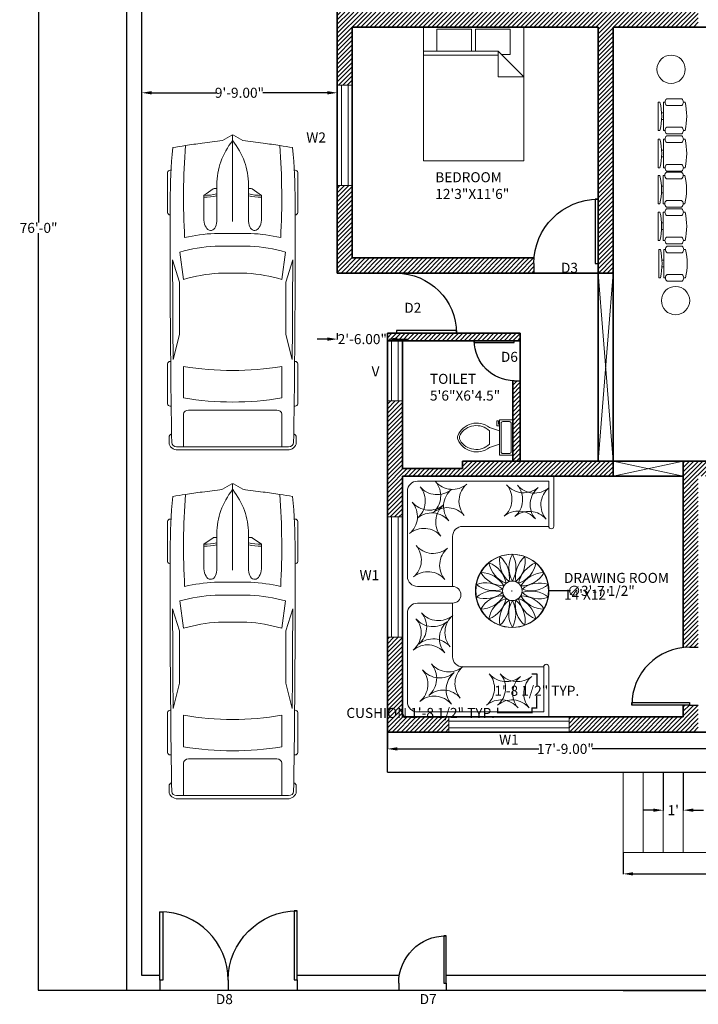
# Model space of a CAD drawing. Units: inches. Extents: x -57 to 1512, y -896 to 149.
# Tile 1 of 6: x -57 to 349, y -896 to -307. Entities that reach past the tile are written whole.
import ezdxf

# ---------------------------------------------------------------- set-up
doc = ezdxf.new("R2010")
doc.units = ezdxf.units.IN
doc.header["$MEASUREMENT"] = 0
doc.layers.get('Defpoints').update_dxf_attribs({"color": 9})
for name, color, linetype, lineweight in [('A-ANNO-DIMS', 2, 'Continuous', 18), ('A-ANNO-TEXT', 7, 'Continuous', 18), ('A-AREA-IDEN', 7, 'Continuous', 18), ('A-DOOR', 3, 'Continuous', 25), ('A-FLOR', 7, 'Continuous', 25), ('A-FLOR-FIXT', 9, 'Continuous', 18), ('A-FLOR-STRS', 7, 'Continuous', 18), ('A-FURN', 8, 'Continuous', 18), ('A-GLAZ', 4, 'Continuous', 18), ('A-WALL', 7, 'Continuous', 35), ('A-WALL-OPEN', 7, 'Continuous', 18), ('A-WALL-PATT', 8, 'Continuous', 13), ('C-PROP', 7, 'Continuous', 25), ('car', 250, 'Continuous', 18), ('L-SITE-GATE', 3, 'Continuous', 25)]:
    doc.layers.add(name, color=color, linetype=linetype, lineweight=lineweight)
doc.styles.get("Standard").update_dxf_attribs({"font": 'arial.ttf'})
doc.dimstyles.get("Standard").update_dxf_attribs({"dimtxt": 6, "dimasz": 0.18, "dimexe": 0.18, "dimexo": 0.0625, "dimgap": 0.09, "dimtad": 0, "dimtih": 1, "dimtoh": 1, "dimzin": 0, "dimdsep": 46, "dimlunit": 3, "dimtxsty": 'Standard', "dimcen": 0.09, "dimadec": 0, "dimazin": 0, "dimtfac": 1, "dimtofl": 0, "dimtmove": 0, "dimatfit": 3, "dimfxl": 1, "dimtolj": 1, "dimtzin": 0, "dimarcsym": 0})

# ---------------------------------------------------------------- blocks, each defined once
blk = doc.blocks.new('*U2')
for p, q in [((0, 0), (0, -6)), ((40, 0), (40, -6))]:
    blk.add_line(p, q)
blk.add_lwpolyline([(0, 0), (0, 40), (1.75, 40), (1.75, 0)], close=True)
blk.add_arc((0, 0), 40, 0, 90)
blk = doc.blocks.new('*U3')
for radius in [21.87, 5.87]:
    blk.add_circle((21.87, 21.87), radius)
for centre, radius, start, end in [((36.4, 35.73), 16.59, 151.17306, 208.82694), ((8.19, 35.73), 15.84, 329.67427, 30.32573)]:
    blk.add_arc(centre, radius, start, end)
blk = doc.blocks.new('*U4')
at = {"layer": 'A-FURN', "color": 0, "linetype": 'ByBlock', "lineweight": -2, "transparency": 16777216}
for p, rotation in [((-154.62, -679.14), 39.99999999999997), ((-121.11, -645.64), 139.9999999999998), ((-149.23, -617.53), 219.9999999999997), ((-182.73, -651.03), 319.9999999999997), ((-143.92, -678.21), 59.99999999999992), ((-122.05, -656.34), 119.9999999999998), ((-159.92, -618.47), 239.9999999999997), ((-181.79, -640.33), 299.9999999999996), ((-164.99, -676.36), 19.99999999999997), ((-123.89, -635.27), 159.9999999999999), ((-138.85, -620.31), 199.9999999999997), ((-179.95, -661.41), 339.9999999999997), ((-134.18, -673.67), 79.99999999999991), ((-126.59, -666.07), 99.99999999999984), ((-169.66, -623.01), 259.9999999999997), ((-177.25, -630.6), 279.9999999999997), ((-130.05, -626.47), 180)]:
    blk.add_blockref('*U3', p, dxfattribs=dict(at, rotation=rotation))
blk.add_blockref('*U3', (-173.79, -670.2), dxfattribs=at)
blk = doc.blocks.new('Bed - Queen')
for p, q in [((0, -80.00003), (0, 0)), ((0, 0), (59.99999, 0)), ((59.99999, 0), (59.99999, -80.00003)), ((7.99999, -1.2), (28.79998, -1.2)), ((7.99999, -14.4), (7.99999, -1.2)), ((28.79998, -1.2), (28.79998, -14.4)), ((31.19999, -1.2), (51.99999, -1.2)), ((31.19999, -14.4), (31.19999, -1.2)), ((51.99999, -1.2), (51.99999, -16.4)), ((0, -14.4), (44.8, -14.4)), ((44.8, -16.8), (0, -16.8)), ((59.99999, -29.6), (44.8, -14.4)), ((44.8, -14.4), (44.8, -29.6)), ((51.99999, -16.4), (46.79936, -16.4)), ((44.8, -29.6), (59.99999, -29.6)), ((59.99999, -80.00003), (0, -80.00003))]:
    blk.add_line(p, q)
blk = doc.blocks.new('Chair - Desk')
for p, q in [((-8.5, 0), (-8.5, -1)), ((-8.5, 0), (8.5, 0)), ((8.5, 0), (8.5, -1)), ((-10.5, -5), (-10.5, -14)), ((-8.5, -3), (-8.5, -4)), ((-8.5, -3), (8.5, -3)), ((-6.5, -14), (-6.5, -5)), ((-2, -3), (-2, -1.9355)), ((2, -1.9576), (2, -3)), ((6.5, -5), (6.5, -14)), ((8.5, -3), (8.5, -4)), ((10.5, -14), (10.5, -5)), ((-8.5, -15), (-8.5, -16)), ((8.5, -15), (8.5, -16))]:
    blk.add_line(p, q)
for centre, radius, start, end in [((-8.5, -6.5), 2.5, 36.8699, 143.1301), ((0, 34.625), 36.625, 256.5803, 283.4197), ((8.5, -6.5), 2.5, 36.8699, 143.1301), ((-8.5, -12.5), 2.5, 216.8699, 323.1301), ((0, 19.625), 36.625, 256.5803, 283.4197), ((8.5, -12.5), 2.5, 216.8699, 323.1301)]:
    blk.add_arc(centre, radius, start, end)
blk = doc.blocks.new('*D13')
at = {"layer": 'A-ANNO-DIMS', "color": 0, "lineweight": -2, "transparency": 16777216}
for p, q in [((163.3, -732.82), (163.3, -743.03)), ((376.3, -732.82), (376.3, -743.03)), ((169.3, -742.85), (253.86, -742.85)), ((370.3, -742.85), (285.74, -742.85))]:
    blk.add_line(p, q, dxfattribs=at)
at = {"layer": 'A-ANNO-DIMS', "color": 0, "transparency": 16777216}
for points in [[(169.3, -741.85), (169.3, -743.85), (163.3, -742.85)], [(370.3, -741.85), (370.3, -743.85), (376.3, -742.85)]]:
    blk.add_solid(points, dxfattribs=at)
at = {"layer": 'Defpoints', "color": 0, "transparency": 16777216}
for p in [(163.3, -732.76), (376.3, -732.76), (376.3, -742.85)]:
    blk.add_point(p, dxfattribs=at)
at = {"layer": 'A-ANNO-DIMS', "color": 0, "transparency": 16777216, "insert": (269.8, -742.85), "char_height": 6, "attachment_point": 5}
blk.add_mtext('\\A1;17\'-9.00"', dxfattribs=at)
blk = doc.blocks.new('*D14')
at = {"layer": 'A-ANNO-DIMS', "color": 0, "lineweight": -2, "transparency": 16777216}
for p, q in [((304.3, -804.82), (304.3, -817.78)), ((520.3, -804.82), (520.3, -817.78)), ((310.3, -817.6), (407.4, -817.6)), ((514.3, -817.6), (417.19, -817.6))]:
    blk.add_line(p, q, dxfattribs=at)
at = {"layer": 'A-ANNO-DIMS', "color": 0, "transparency": 16777216}
for points in [[(310.3, -816.6), (310.3, -818.6), (304.3, -817.6)], [(514.3, -816.6), (514.3, -818.6), (520.3, -817.6)]]:
    blk.add_solid(points, dxfattribs=at)
at = {"layer": 'Defpoints', "color": 0, "transparency": 16777216}
for p in [(304.3, -804.76), (520.3, -804.76), (520.3, -817.6)]:
    blk.add_point(p, dxfattribs=at)
at = {"layer": 'A-ANNO-DIMS', "color": 0, "transparency": 16777216, "insert": (412.3, -817.6), "char_height": 6, "attachment_point": 5}
blk.add_mtext("\\A1;18'", dxfattribs=at)
blk = doc.blocks.new('*D15')
at = {"layer": 'A-ANNO-DIMS', "color": 0, "lineweight": -2, "transparency": 16777216}
for p, q in [((328.3, -756.82), (328.3, -779.69)), ((340.3, -756.82), (340.3, -779.69)), ((322.3, -779.51), (316.3, -779.51)), ((346.3, -779.51), (352.3, -779.51))]:
    blk.add_line(p, q, dxfattribs=at)
at = {"layer": 'A-ANNO-DIMS', "color": 0, "transparency": 16777216}
for points in [[(322.3, -778.51), (322.3, -780.51), (328.3, -779.51)], [(346.3, -778.51), (346.3, -780.51), (340.3, -779.51)]]:
    blk.add_solid(points, dxfattribs=at)
at = {"layer": 'Defpoints', "color": 0, "transparency": 16777216}
for p in [(328.3, -756.76), (340.3, -756.76), (340.3, -779.51)]:
    blk.add_point(p, dxfattribs=at)
at = {"layer": 'A-ANNO-DIMS', "color": 0, "transparency": 16777216, "insert": (334.3, -779.51), "char_height": 6, "attachment_point": 5}
blk.add_mtext("\\A1;1'", dxfattribs=at)
blk = doc.blocks.new('*D17')
at = {"layer": 'A-ANNO-DIMS', "color": 0, "lineweight": -2, "transparency": 16777216}
for p, q in [((133.3, -494.32), (133.3, -497.97)), ((163.3, -494.32), (163.3, -497.97)), ((127.3, -497.79), (121.3, -497.79)), ((169.3, -497.79), (175.3, -497.79))]:
    blk.add_line(p, q, dxfattribs=at)
at = {"layer": 'A-ANNO-DIMS', "color": 0, "transparency": 16777216}
for points in [[(127.3, -496.79), (127.3, -498.79), (133.3, -497.79)], [(169.3, -496.79), (169.3, -498.79), (163.3, -497.79)]]:
    blk.add_solid(points, dxfattribs=at)
at = {"layer": 'Defpoints', "color": 0, "transparency": 16777216}
for p in [(133.3, -494.26), (163.3, -494.26), (133.3, -497.79)]:
    blk.add_point(p, dxfattribs=at)
at = {"layer": 'A-ANNO-DIMS', "color": 0, "transparency": 16777216, "insert": (148.3, -497.79), "char_height": 6, "attachment_point": 5}
blk.add_mtext('\\A1;2\'-6.00"', dxfattribs=at)
blk = doc.blocks.new('*D19')
at = {"layer": 'A-ANNO-DIMS', "color": 0, "lineweight": -2, "transparency": 16777216}
for p, q in [((16.3, -302.32), (16.3, -350.65)), ((133.3, -302.32), (133.3, -350.65)), ((22.3, -350.47), (60.91, -350.47)), ((127.3, -350.47), (88.69, -350.47))]:
    blk.add_line(p, q, dxfattribs=at)
at = {"layer": 'A-ANNO-DIMS', "color": 0, "transparency": 16777216}
for points in [[(22.3, -349.47), (22.3, -351.47), (16.3, -350.47)], [(127.3, -349.47), (127.3, -351.47), (133.3, -350.47)]]:
    blk.add_solid(points, dxfattribs=at)
at = {"layer": 'Defpoints', "color": 0, "transparency": 16777216}
for p in [(16.3, -302.26), (133.3, -302.26), (16.3, -350.47)]:
    blk.add_point(p, dxfattribs=at)
at = {"layer": 'A-ANNO-DIMS', "color": 0, "transparency": 16777216, "insert": (74.8, -350.47), "char_height": 6, "attachment_point": 5}
blk.add_mtext('\\A1;9\'-9.00"', dxfattribs=at)
blk = doc.blocks.new('*U24')
for p, q in [((9.5, -6), (9.5, -2)), ((-10, -8.5), (-8, -8.5)), ((-10, -9.5), (-10, -8.5)), ((-7, -9.5), (-10, -9.5)), ((-8, -8.5), (-8, -8)), ((-7, -8), (-7, -9.5)), ((-4, -8), (-6, -14)), ((4, -8), (6, -14)), ((4, -14), (-4, -14))]:
    blk.add_line(p, q)
blk.add_lwpolyline([(10.5, -8), (10.5, 0), (-10.5, 0), (-10.5, -8)], close=True)
for points in [[(-9.5, -2), (-9.5, -6)], [(8.5, -1), (-8.5, -1)], [(-8.5, -7), (8.5, -7)]]:
    blk.add_lwpolyline(points)
for centre, radius, start, end in [((-8.62, -1.88), 0.884, 81.8699, 188.1301), ((8.62, -1.88), 0.884, 351.8699, 98.1301), ((-8.62, -6.12), 0.884, 171.8699, 278.1301), ((8.62, -6.12), 0.884, 261.8699, 8.1301), ((3.52, -21.58), 12.17, 141.46911, 247.97143), ((4.2, -21.82), 11.33, 136.36773, 238.94682), ((-3.52, -21.58), 12.17, 292.02843, 38.53071), ((-4.2, -21.82), 11.33, 301.05301, 43.63209), ((0, -27.88), 4, 245.73182, 294.26817), ((0, -29), 4, 254.86053, 285.13947)]:
    blk.add_arc(centre, radius, start, end)
blk = doc.blocks.new('*U22')
for p, q in [((21.1, 37.41), (21.1, 36.83)), ((46.55, 38.89), (22.35, 38.89)), ((47.8, 37.39), (47.8, 37.41)), ((87.99, 31.87), (74.76, 35.92)), ((134.31, 35.6), (119.29, 31.78)), ((135.45, 37.07), (135.45, 37.41)), ((136.7, 38.89), (160.9, 38.89)), ((162.15, 37.41), (162.15, 36.77)), ((70.03, 31.54), (86.41, 29.35)), ((186.47, -33.5), (186.47, 33.5)), ((188.4, -32.76), (188.4, 32.76)), ((138.42, 29.35), (157.25, 29.35)), ((164.52, 26.39), (164.52, -26.39)), ((186.47, 29.35), (167.01, 29.35)), ((32.27, 11.63), (36.13, 17.17)), ((36.13, 17.17), (50.94, 17.17)), ((3.27, 6.13), (0.1, 0.41)), ((29.77, 9.51), (51.68, 9.51)), ((32.12, 9.51), (32.12, 11.15)), ((58.92, -10.77), (58.92, 10.77)), ((66.55, -10.53), (66.55, 10.53)), ((82.74, 8.5), (82.74, -8.5)), ((186.47, -10.53), (186.47, 10.53)), ((0, 0), (51.68, 0)), ((0.1, -0.41), (3.27, -6.13)), ((29.77, -9.51), (51.68, -9.51)), ((32.12, -9.51), (32.12, -11.15)), ((32.27, -11.63), (36.13, -17.17)), ((36.13, -17.17), (50.94, -17.17)), ((86.41, -29.35), (70.03, -31.54)), ((157.25, -29.35), (138.42, -29.35)), ((167.01, -29.35), (186.47, -29.35)), ((87.99, -31.87), (74.76, -35.92)), ((134.31, -35.6), (119.29, -31.78)), ((21.1, -37.41), (21.1, -36.83)), ((46.55, -38.89), (22.35, -38.89)), ((47.8, -37.39), (47.8, -37.41)), ((135.45, -37.07), (135.45, -37.41)), ((136.7, -38.89), (160.9, -38.89)), ((162.15, -37.41), (162.15, -36.77))]:
    blk.add_line(p, q)
for centre, major_axis, ratio, start_param, end_param in [((266.03, -27.52), (0, 313.31), 0.842304, 1.367076, 1.39176), ((41.19, -490.86), (0, 528.23), 0.842304, 0.00281, 0.075598), ((22.35, 37.41), (0, -1.48), 0.842304, 3.141593, 4.712389), ((64.48, -10555.62), (0, 10593.03), 0.842304, -0.013397, 0.002797), ((46.55, 37.41), (0, 1.48), 0.842304, -1.570796, 0), ((64.48, -10555.62), (0, -10591.55), 0.842304, 3.133765, 3.140441), ((136.7, 37.41), (0, -1.48), 0.842304, 3.141593, 4.712389), ((160.9, 37.41), (0, 1.48), 0.842304, -1.570796, 0), ((180.63, 35.84), (0, 2.22), 0.842304, -0.013017, 1.249894), ((64.48, -10556.36), (0, 10595.31), 0.842304, -0.013397, -0.013017), ((183.98, 33.5), (0, -2.96), 0.842304, 1.570796, 3.128196), ((183.98, 32.76), (0, -5.25), 0.842304, 1.570796, 3.128196), ((37.47, -593.96), (0, -623.33), 0.842304, 3.096046, 3.200911), ((135.29, 5.39), (0, 81.77), 0.842304, 1.245306, 1.50788), ((95.79, -3666.35), (0, -3698.24), 0.842304, 3.134049, 3.144098), ((259.18, -27.52), (0, -305.3), 0.842304, 4.528606, 4.561838), ((134.4, 5.39), (0, -89.78), 0.842304, 4.449482, 4.652344), ((149.6, 2.8), (0, -79.58), 0.842304, 4.372215, 4.640744), ((17.08, 0), (0, 147.02), 0.842304, 4.511394, 4.913384), ((35.91, 0), (0, 147.02), 0.842304, 4.511394, 4.913384), ((167.01, 26.39), (0, 2.96), 0.842304, 0, 1.570796), ((-204.49, 52.4), (0, -250.96), 0.842304, 1.385369, 1.434372), ((13.04, 17.01), (0, 27.42), 0.842304, 4.435146, 4.718221), ((14.2, 17.01), (0, 27.42), 0.842304, 4.435146, 4.718221), ((50.79, 13.34), (6.34, -0.36), 0.603834, -1.395552, 1.581315), ((29.77, -46.66), (0, 56.17), 0.842304, 0, 0.590319), ((32.75, 11.15), (0, 0.74), 0.842304, 0.879714, 1.570796), ((0.62, 0), (0, -0.74), 0.842304, 4.131459, 5.293319), ((29.77, 46.66), (0, 56.17), 0.842304, 2.551274, 3.141593), ((-204.49, -52.4), (0, 250.96), 0.842304, -1.434372, -1.385369), ((32.75, -11.15), (0, -0.74), 0.842304, 4.712389, 5.403472), ((13.04, -17.01), (0, -27.42), 0.842304, 1.564964, 1.848039), ((14.2, -17.01), (0, -27.42), 0.842304, 1.564964, 1.848039), ((134.4, -5.39), (0, -89.78), 0.842304, -1.510751, -1.307889), ((135.29, -5.39), (0, -81.77), 0.842304, -1.50788, -1.245306), ((149.6, -2.8), (0, -79.58), 0.842304, -1.499151, -1.230623), ((259.18, 27.52), (0, 305.3), 0.842304, 1.721348, 1.754579), ((266.03, 27.52), (0, 313.31), 0.842304, 1.749832, 1.774517), ((37.47, 593.96), (0, -623.33), 0.842304, -0.059319, 0.045547), ((167.01, -26.39), (0, -2.96), 0.842304, 4.712389, 6.283185), ((95.79, 3666.35), (0, -3698.24), 0.842304, -0.002505, 0.007544), ((183.98, -33.5), (0, 2.96), 0.842304, 3.15499, 4.712389), ((183.98, -32.76), (0, -5.25), 0.842304, 0.013397, 1.570796), ((41.19, 490.86), (0, -528.23), 0.842304, -0.075598, -0.00281), ((22.35, -37.41), (0, 1.48), 0.842304, 1.570796, 3.141593), ((64.48, 10555.62), (0, 10593.03), 0.842304, 3.138796, 3.15499), ((46.55, -37.41), (0, -1.48), 0.842304, 0, 1.570796), ((64.48, 10555.62), (0, -10591.55), 0.842304, 0.001152, 0.007828), ((136.7, -37.41), (0, -1.48), 0.842304, -1.570796, 0), ((160.9, -37.41), (0, 1.48), 0.842304, 3.141593, 4.712389), ((180.63, -35.84), (0, -2.22), 0.842304, -1.249894, 0.013017), ((64.48, 10556.36), (0, 10595.31), 0.842304, 3.15461, 3.15499)]:
    blk.add_ellipse(centre, major_axis=major_axis, ratio=ratio, start_param=start_param, end_param=end_param)
at = {"extrusion": (0, 0, -1)}
blk.add_ellipse((50.79, -13.34), major_axis=(6.34, 0.36), ratio=0.603834, start_param=-1.395552, end_param=1.581315, dxfattribs=at)
blk = doc.blocks.new('GLAZ-SASH-36IN')
for p, q in [((0, 4), (36, 4)), ((0, 0), (36, 0))]:
    blk.add_line(p, q)
blk = doc.blocks.new('WIN-60IN')
for p, q in [((0, 60), (9, 60)), ((2.5, 60), (2.5, 0)), ((6.5, 60), (6.5, 0)), ((0, 0), (9, 0))]:
    blk.add_line(p, q)
blk = doc.blocks.new('WIN-72IN')
for p, q in [((0, 0), (0, 9)), ((0, 6.5), (72, 6.5)), ((72, 0), (72, 9)), ((0, 2.5), (72, 2.5))]:
    blk.add_line(p, q)
blk = doc.blocks.new('SOFA-CUSHION')
blk.add_lwpolyline([(20.39, 18.8, 0.414214), (18.8, 0, 0.414214), (0, 1.59, 0.414214), (1.59, 20.39, 0.414214)], format="xyb", close=True)
blk = doc.blocks.new('*D91')
at = {"layer": 'A-ANNO-DIMS', "color": 0, "lineweight": -2, "transparency": 16777216}
for p, q in [((229.23, -718.36), (229.23, -721.53)), ((249.62, -718.36), (249.62, -721.53)), ((229.23, -721.35), (229.05, -721.35)), ((249.44, -721.35), (229.41, -721.35))]:
    blk.add_line(p, q, dxfattribs=at)
at = {"layer": 'A-ANNO-DIMS', "color": 0, "transparency": 16777216}
for points in [[(229.41, -721.32), (229.41, -721.38), (229.23, -721.35)], [(249.44, -721.32), (249.44, -721.38), (249.62, -721.35)]]:
    blk.add_solid(points, dxfattribs=at)
at = {"layer": 'Defpoints', "color": 0, "transparency": 16777216}
for p in [(229.23, -718.3), (249.62, -718.3), (229.23, -721.35)]:
    blk.add_point(p, dxfattribs=at)
at = {"layer": 'A-ANNO-DIMS', "color": 0, "transparency": 16777216, "insert": (183.23, -721.35), "char_height": 6, "attachment_point": 5}
blk.add_mtext('\\A1;CUSHION 1\'-8 1/2" TYP.', dxfattribs=at)
blk = doc.blocks.new('*D92')
at = {"layer": 'A-ANNO-DIMS', "color": 0, "lineweight": -2, "transparency": 16777216}
for p, q in [((249.68, -697.91), (252.86, -697.91)), ((252.68, -698.09), (252.68, -704.91)), ((252.68, -718.12), (252.68, -711.29)), ((249.68, -718.3), (252.86, -718.3))]:
    blk.add_line(p, q, dxfattribs=at)
at = {"layer": 'A-ANNO-DIMS', "color": 0, "transparency": 16777216}
for points in [[(252.65, -698.09), (252.71, -698.09), (252.68, -697.91)], [(252.65, -718.12), (252.71, -718.12), (252.68, -718.3)]]:
    blk.add_solid(points, dxfattribs=at)
at = {"layer": 'Defpoints', "color": 0, "transparency": 16777216}
for p in [(249.62, -697.91), (249.62, -718.3), (252.68, -718.3)]:
    blk.add_point(p, dxfattribs=at)
at = {"layer": 'A-ANNO-DIMS', "color": 0, "transparency": 16777216, "insert": (252.68, -708.1), "char_height": 6, "attachment_point": 5}
blk.add_mtext('\\A1;1\'-8 1/2" TYP.', dxfattribs=at)
blk = doc.blocks.new('*D103')
at = {"layer": 'A-ANNO-DIMS', "color": 0, "lineweight": -2, "transparency": 16777216}
for p, q in [((7.23, 24.74), (-45.53, 24.74)), ((-45.35, 24.56), (-45.35, -428.11)), ((-45.35, -887.08), (-45.35, -434.41)), ((7.23, -887.26), (-45.53, -887.26))]:
    blk.add_line(p, q, dxfattribs=at)
at = {"layer": 'A-ANNO-DIMS', "color": 0, "transparency": 16777216}
for points in [[(-45.38, 24.56), (-45.32, 24.56), (-45.35, 24.74)], [(-45.38, -887.08), (-45.32, -887.08), (-45.35, -887.26)]]:
    blk.add_solid(points, dxfattribs=at)
at = {"layer": 'Defpoints', "color": 0, "transparency": 16777216}
for p in [(-45.35, 24.74), (7.3, 24.74), (7.3, -887.26)]:
    blk.add_point(p, dxfattribs=at)
at = {"layer": 'A-ANNO-DIMS', "color": 0, "transparency": 16777216, "insert": (-45.35, -431.26), "char_height": 6, "attachment_point": 5}
blk.add_mtext('\\A1;76\'-0"', dxfattribs=at)
blk = doc.blocks.new('*D108')
at = {"layer": 'A-ANNO-DIMS', "color": 0, "lineweight": -2, "transparency": 16777216}
for p, q in [((237.72, -648.34), (237.9, -648.34)), ((237.81, -648.43), (237.81, -648.25)), ((272.79, -648.34), (259.85, -648.34))]:
    blk.add_line(p, q, dxfattribs=at)
at = {"layer": 'A-ANNO-DIMS', "color": 0, "transparency": 16777216}
blk.add_solid([(259.85, -648.31), (259.85, -648.37), (259.67, -648.34)], dxfattribs=at)
at = {"layer": 'Defpoints', "color": 0, "transparency": 16777216}
for p in [(215.94, -648.34), (259.67, -648.34)]:
    blk.add_point(p, dxfattribs=at)
at = {"layer": 'A-ANNO-DIMS', "color": 0, "transparency": 16777216, "insert": (291.11, -648.34), "char_height": 6, "attachment_point": 5}
blk.add_mtext('\\A1;∅3\'-7 1/2"', dxfattribs=at)

msp = doc.modelspace()

# ---------------------------------------------------------------- hatches: boundary and pattern name
at = {"layer": 'A-WALL-PATT'}
h = msp.add_hatch(dxfattribs=at)
h.set_pattern_fill('ANSI31', color=256, scale=15)
h.paths.add_polyline_path([(496.296, -570.76), (487.296, -570.76), (474.037, -570.76), (474.037, -579.76), (487.296, -579.76), (487.296, -732.76), (545.372, -732.76), (545.372, -723.76), (496.296, -723.76)])
h.paths.add_polyline_path([(661.296, -684.034), (652.296, -684.034), (652.296, -723.76), (617.372, -723.76), (617.372, -732.76), (661.296, -732.76)])
h.paths.add_polyline_path([(298.296, -570.76), (208.296, -570.76), (208.296, -575.26), (172.296, -575.26), (172.296, -534.76), (163.296, -534.76), (163.296, -604.062), (172.296, -604.062), (172.296, -579.76), (298.296, -579.76)])
h.paths.add_polyline_path([(172.296, -494.26), (163.296, -494.26), (163.296, -498.76), (172.296, -498.76)])
h.paths.add_polyline_path([(242.796, -494.26), (172.296, -494.26), (172.296, -498.76), (238.296, -498.76), (242.796, -498.76)])
h.paths.add_polyline_path([(242.796, -522.76), (238.296, -522.76), (238.296, -570.76), (242.796, -570.76)])
h.paths.add_polyline_path([(142.296, -405.989), (133.296, -405.989), (133.296, -458.26), (250.953, -458.26), (250.953, -452.508, -0.0212094), (251.091, -449.26), (142.296, -449.26)])
h.paths.add_polyline_path([(298.296, -311.26), (349.296, -311.26), (349.296, -302.26), (345.753, -302.26), (322.135, -302.26), (133.296, -302.26), (133.296, -345.989), (142.296, -345.989), (142.296, -311.26), (289.296, -311.26), (289.296, -458.26), (298.296, -458.26)])
h.paths.add_polyline_path([(172.296, -275.26), (163.296, -275.26), (163.296, -302.26), (172.296, -302.26)])
h.paths.add_polyline_path([(172.296, -158.26), (230.655, -158.26), (230.655, -149.26), (163.296, -149.26), (163.296, -215.26), (172.296, -215.26)])
h.paths.add_polyline_path([(378.235, -149.26), (266.655, -149.26), (266.655, -158.26), (378.235, -158.26)])
h.paths.add_polyline_path([(349.296, -158.26), (340.296, -158.26), (340.296, -279.28, -0.0583572), (345.753, -278.641), (349.296, -278.641)])
h.paths.add_polyline_path([(529.979, -149.26), (450.235, -149.26), (450.235, -158.26), (529.979, -158.26)])
h.paths.add_polyline_path([(496.296, -158.26), (487.296, -158.26), (487.296, -278.641), (490.839, -278.641, -0.0583572), (496.296, -279.28)])
h.paths.add_polyline_path([(631.296, -149.26), (589.979, -149.26), (589.979, -158.26), (622.296, -158.26), (622.296, -215.26), (631.296, -215.26)])
h.paths.add_polyline_path([(661.296, -302.26), (631.296, -302.26), (631.296, -275.26), (622.296, -275.26), (622.296, -302.26), (487.296, -302.26), (487.296, -458.26), (496.296, -458.26), (496.296, -453.783), (496.296, -423.936), (496.296, -311.26), (652.296, -311.26), (652.296, -340.453), (661.296, -340.453)])
h.paths.add_polyline_path([(349.296, -579.76), (359.066, -579.76), (359.066, -570.76), (340.296, -570.76), (340.296, -682.249, -0.0275619), (344.104, -682.039), (349.296, -682.039)])
h.paths.add_polyline_path([(172.296, -676.062), (163.296, -676.062), (163.296, -732.76), (200.083, -732.76), (200.083, -723.76), (172.296, -723.76)])
h.paths.add_polyline_path([(349.296, -716.654), (344.104, -716.654), (340.296, -716.654), (340.296, -723.76), (272.083, -723.76), (272.083, -732.76), (349.296, -732.76)])

# ---------------------------------------------------------------- linework, layer by layer
at = {"layer": 'A-FLOR'}
for q in [(163.296, -732.76), (376.296, -756.76)]:
    msp.add_line((163.296, -756.76), q, dxfattribs=at)
at = {"layer": 'A-FLOR-STRS'}
for p, q in [((304.296, -804.76), (304.296, -756.76)), ((316.296, -804.76), (316.296, -756.76)), ((328.296, -804.76), (328.296, -756.76)), ((340.296, -804.76), (340.296, -756.76)), ((304.296, -804.76), (520.296, -804.76))]:
    msp.add_line(p, q, dxfattribs=at)
at = {"layer": 'A-FURN'}
for p, q in [((181.296, -582.76), (259.845, -582.76)), ((259.845, -582.76), (259.845, -609.76)), ((262.845, -579.76), (262.845, -609.76)), ((175.296, -588.76), (175.296, -639.704)), ((208.296, -609.76), (259.845, -609.76)), ((202.296, -615.76), (202.296, -645.704)), ((202.296, -645.704), (181.296, -645.704)), ((202.296, -655.704), (181.296, -655.704)), ((202.296, -655.704), (202.296, -687.76)), ((175.296, -661.704), (175.296, -714.76)), ((208.296, -693.76), (256.845, -693.76)), ((256.845, -693.76), (256.845, -720.76)), ((259.845, -693.76), (259.845, -723.76)), ((181.296, -720.76), (256.845, -720.76))]:
    msp.add_line(p, q, dxfattribs=at)
for centre, radius in [((333.025, -336.407), 8.464), ((335.671, -474.764), 8.464), ((237.808, -648.338), 21.866)]:
    msp.add_circle(centre, radius, dxfattribs=at)
for centre, radius, start, end in [((181.296, -588.76), 6, 90, 180), ((208.296, -615.76), 6, 90, 180), ((261.345, -609.76), 1.5, 180, 0), ((181.296, -639.704), 6, 180, 270), ((202.296, -650.704), 5, 270, 90), ((181.296, -661.704), 6, 90, 180), ((208.296, -687.76), 6, 180, 270), ((258.345, -693.76), 1.5, 0, 180), ((181.296, -714.76), 6, 180, 270)]:
    msp.add_arc(centre, radius, start, end, dxfattribs=at)
at = {"layer": 'A-GLAZ'}
msp.add_line((163.296, -534.76), (172.296, -534.76), dxfattribs=at)
at = {"layer": 'A-WALL'}
for p, q in [((133.296, -302.26), (133.296, -458.26)), ((142.296, -311.26), (289.296, -311.26)), ((142.296, -311.26), (142.296, -449.26)), ((289.296, -311.26), (289.296, -570.76)), ((298.296, -311.26), (298.296, -579.76)), ((298.296, -311.26), (487.296, -311.26)), ((142.296, -449.26), (251.091, -449.26)), ((133.296, -458.26), (298.296, -458.26)), ((163.296, -494.26), (242.796, -494.26)), ((163.296, -494.26), (163.296, -732.76)), ((242.796, -494.26), (242.796, -570.76)), ((163.296, -498.76), (238.296, -498.76)), ((172.296, -498.76), (172.296, -575.26)), ((172.296, -498.76), (172.296, -575.26)), ((242.796, -498.76), (238.296, -498.76)), ((238.296, -522.656), (238.296, -570.76)), ((208.296, -570.76), (391.277, -570.76)), ((208.296, -570.76), (208.296, -575.26)), ((340.296, -570.76), (340.296, -682.249)), ((172.296, -575.26), (208.296, -575.26)), ((172.296, -579.76), (340.296, -579.76)), ((172.296, -579.76), (172.296, -723.76)), ((340.296, -716.654), (340.296, -723.76)), ((172.296, -723.76), (340.296, -723.76)), ((172.296, -723.76), (340.296, -723.76)), ((163.296, -732.76), (376.296, -732.76))]:
    msp.add_line(p, q, dxfattribs=at)
at = {"layer": 'A-WALL-OPEN'}
for p, q in [((289.296, -458.26), (298.296, -570.76)), ((289.296, -570.76), (298.296, -458.26)), ((298.296, -579.76), (340.296, -570.76)), ((298.296, -570.76), (340.296, -579.76))]:
    msp.add_line(p, q, dxfattribs=at)
at = {"layer": 'C-PROP'}
for p, q in [((7.296, 24.74), (7.296, -887.26)), ((16.296, -302.26), (16.296, -458.26)), ((16.296, -458.26), (16.296, -878.26)), ((16.296, -878.26), (27.213, -878.26)), ((67.971, -878.26), (68.167, -878.26)), ((109.395, -878.26), (170.45, -878.26)), ((198.4, -878.26), (600.465, -878.26)), ((712.296, -887.26), (7.296, -887.26)), ((304.296, -887.26), (520.296, -887.26))]:
    msp.add_line(p, q, dxfattribs=at)

# ---------------------------------------------------------------- block references
at = {"layer": 'A-DOOR', "xscale": -0.9585752359828884, "yscale": 0.9585752359828884, "zscale": 0.9585752359828884}
msp.add_blockref('*U2', (289.296, -452.508), dxfattribs=at)
at = {"layer": 'A-DOOR'}
for p, xscale, yscale, zscale, rotation in [((168.68, -494.26), -0.8973103668394152, 0.8973103668394152, 0.8973103668394152, 270), ((239.209, -498.76), -0.5978360704994329, 0.5978360704994329, 0.5978360704994329, 90), ((344.104, -716.654), 0.8653953225033477, 0.8653953225033477, 0.8653953225033477, 90.00000000000003)]:
    msp.add_blockref('*U2', p, dxfattribs=dict(at, xscale=xscale, yscale=yscale, zscale=zscale, rotation=rotation))
at = {"layer": 'A-FLOR-FIXT', "rotation": 270}
msp.add_blockref('*U24', (238.296, -556.645), dxfattribs=at)
at = {"layer": 'A-FURN'}
for name, p in [('Bed - Queen', (184.825, -311.26)), ('SOFA-CUSHION', (239.46, -605.528)), ('*U4', (389.979, 0))]:
    msp.add_blockref(name, p, dxfattribs=at)
for name, p, rotation in [('Chair - Desk', (325.375, -364.518), 90), ('Chair - Desk', (325.375, -386.785), 90), ('Chair - Desk', (325.261, -408.359), 90), ('Chair - Desk', (325.355, -430.289), 90), ('Chair - Desk', (325.598, -452.621), 90), ('SOFA-CUSHION', (210.868, -582.928), 180), ('SOFA-CUSHION', (201.632, -586.058), 180), ('SOFA-CUSHION', (253.449, -584.967), 180), ('SOFA-CUSHION', (196.928, -595.338), 180), ('SOFA-CUSHION', (199.287, -621.247), 180), ('SOFA-CUSHION', (199.158, -664.984), 180), ('SOFA-CUSHION', (202.454, -661.406), 180), ('SOFA-CUSHION', (208.454, -692.036), 180), ('SOFA-CUSHION', (203.195, -695.672), 180), ('SOFA-CUSHION', (243.021, -697.909), 180), ('SOFA-CUSHION', (249.619, -697.909), 180)]:
    msp.add_blockref(name, p, dxfattribs=dict(at, rotation=rotation))
at = {"layer": 'A-GLAZ'}
for name, p, rotation in [('WIN-60IN', (142.296, -345.989), 180), ('GLAZ-SASH-36IN', (169.796, -534.76), 90.00000000000003), ('WIN-72IN', (163.295, -604.062), 270.0000000000001)]:
    msp.add_blockref(name, p, dxfattribs=dict(at, rotation=rotation))
msp.add_blockref('WIN-72IN', (200.083, -732.76), dxfattribs=at)
at = {"layer": 'car', "rotation": 270}
for p in [(70.738, -375.679), (70.738, -584.321)]:
    msp.add_blockref('*U22', p, dxfattribs=at)
at = {"layer": 'L-SITE-GATE'}
for p, xscale, yscale, zscale in [((27.213, -881.131), 1.021473734565475, 1.021473734565475, 1.021473734565475), ((109.395, -881.061), -1.033061844354514, 1.033061844354514, 1.033061844354514), ((198.4, -883.007), -0.7087727837398609, 0.7087727837398609, 0.7087727837398609)]:
    msp.add_blockref('*U2', p, dxfattribs=dict(at, xscale=xscale, yscale=yscale, zscale=zscale))

# ---------------------------------------------------------------- texts
at = {"layer": 'A-ANNO-TEXT', "char_height": 6, "attachment_point": 1}
for s, heights, insert in [('W2', [0], (114.803, -374.212)), ('D3', [6.131], (267.135, -452.129)), ('D2', [0], (173.388, -476.07)), ('D6', [6.131], (231.191, -505.394)), ('V', [0], (153.842, -514.117)), ('W1', [0], (146.665, -635.956)), ('W1', [0], (230.125, -734.343)), ('D8', [6.131], (60.683, -889.499)), ('D7', [6.131], (182.6, -889.499))]:
    msp.add_mtext_dynamic_manual_height_columns(s, width=173.83392, gutter_width=1, heights=heights, dxfattribs=dict(at, insert=insert))
at = {"layer": 'A-AREA-IDEN', "char_height": 6, "attachment_point": 1}
for s, insert in [('BEDROOM\\P12\'3"X11\'6"', (191.936, -397.969)), ('TOILET\\P5\'6"X6\'4.5"', (188.769, -518.547)), ("DRAWING ROOM\\P14'X12'", (268.951, -637.575))]:
    msp.add_mtext_dynamic_manual_height_columns(s, width=160.11736, gutter_width=1, heights=[0], dxfattribs=dict(at, insert=insert))

# ---------------------------------------------------------------- dimensions: what is measured, and where the dimension line sits
at = {"layer": 'A-ANNO-DIMS'}
dim = msp.add_linear_dim(base=(-45.354, 24.74), p1=(7.296, -887.26), p2=(7.296, 24.74), angle=90, dimstyle='Standard', override={"dimdec": 1, "dimlfac": 1, "dimrnd": 0, "dimzin": 1, "dimdsep": 46, "dimlunit": 4, "dimfrac": 2}, dxfattribs=at)
dim.commit()
dim.dimension.update_dxf_attribs({"geometry": '*D103', "text_midpoint": (-45.354, -431.26)})
for base, p1, p2, picture, middle in [((16.296, -350.472), (133.296, -302.26), (16.296, -302.26), '*D19', (74.796, -350.472)), ((133.296, -497.787), (163.296, -494.26), (133.296, -494.26), '*D17', (148.296, -497.787)), ((376.296, -742.845), (163.296, -732.76), (376.296, -732.76), '*D13', (269.796, -742.845)), ((340.296, -779.512), (328.296, -756.76), (340.296, -756.76), '*D15', (334.296, -779.512)), ((520.296, -817.601), (304.296, -804.76), (520.296, -804.76), '*D14', (412.296, -817.601))]:
    dim = msp.add_linear_dim(base=base, p1=p1, p2=p2, dimstyle='Standard', override={"dimasz": 6, "dimclrd": 0, "dimclre": 0, "dimclrt": 0}, dxfattribs=at)
    dim.commit()
    dim.dimension.update_dxf_attribs({"geometry": picture, "text_midpoint": middle})
dim = msp.add_diameter_dim_2p(p1=(215.942, -648.337), p2=(259.675, -648.338), dimstyle='Standard', override={"dimdec": 1, "dimlfac": 1, "dimrnd": 0, "dimzin": 1, "dimdsep": 46, "dimlunit": 4, "dimfrac": 2}, dxfattribs=at)
dim.commit()
dim.dimension.update_dxf_attribs({"geometry": '*D108', "text_midpoint": (272.795, -648.338), "dimtype": 163})
for base, p1, p2, angle, text, picture, middle in [((252.677, -718.295), (249.619, -697.91), (249.619, -718.295), 270, '<> TYP.', '*D92', (252.677, -708.103)), ((229.234, -721.353), (249.619, -718.295), (229.234, -718.295), 180, 'CUSHION <> TYP.', '*D91', (183.231, -721.353))]:
    dim = msp.add_linear_dim(base=base, p1=p1, p2=p2, angle=angle, text=text, dimstyle='Standard', override={"dimdec": 1, "dimlfac": 1, "dimrnd": 0, "dimzin": 1, "dimdsep": 46, "dimlunit": 4, "dimfrac": 2}, dxfattribs=at)
    dim.commit()
    dim.dimension.update_dxf_attribs({"geometry": picture, "text_midpoint": middle})

doc.saveas('drawing.dxf')
